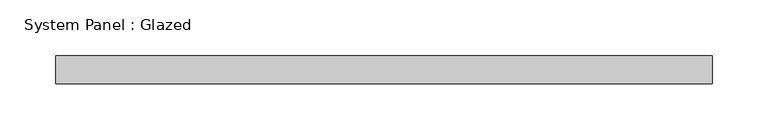
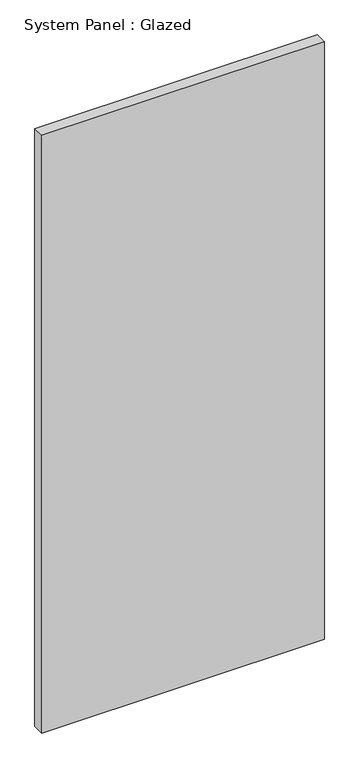
"""IFC4 building model written with IfcOpenShell, lengths in millimetres: plate geometry, System Panel : Glazed."""

from ifc_helpers import new_model, si_unit, origin, origin_with_axes, place, context, project, spatial, polyline, outline, extrude, source, transform, mapped, element, save


def system_panel_glazed_77db913b(model_context):
    return source(origin(), model_context, "Body", "SweptSolid", [
        extrude(outline(polyline([(295.275, 19.05), (-295.275, 19.05), (-295.275, 44.45), (295.275, 44.45), (295.275, 19.05)])), origin_with_axes(), (0.0, 0.0, 1.0), 1320.0507887),
    ])


if __name__ == "__main__":
    model = new_model("IFC4")
    model_context = context("Model", 3, world=origin())
    ifc_project = project(units=[si_unit("LENGTHUNIT", "METRE", prefix="MILLI")], contexts=[model_context])
    site = spatial("IfcSite", under=ifc_project)
    building = spatial("IfcBuilding", under=site)
    placement = place(None, origin())
    system_panel_glazed_shape = system_panel_glazed_77db913b(model_context)
    element("IfcPlate", 1, ObjectType="System Panel : Glazed", at=placement, inside=building, context=model_context, shape_type="MappedRepresentation", body=[
        mapped(system_panel_glazed_shape, transform((0.0, 0.0, 0.0), x_axis=(1.0, 0.0, 0.0), y_axis=(0.0, 1.0, 0.0), z_axis=(0.0, 0.0, 1.0))),
    ])
    save(model, "model.ifc")

# Revit data of these elements
# Type "System Panel : Glazed"
#   Construction Type Id = "GSP4R"
#   Analytic Construction = "1/8 in Pilkington single glazing"
#   Visual Light Transmittance = 0.9
#   Solar Heat Gain Coefficient = 0.86
#   Heat Transfer Coefficient (U) = 1.18115 BTU/(h·ft²·°F)
#   Define Thermal Properties by = 1
# Element 1 (IfcPlate, "System Panel : Glazed")
#   Materials on its faces: "Glass"
# Materials
#   "Glass": class "Glass", colour RGB 0 128 192, transparency 0.75, Description = "Soda Lime Glass", Cost = 0
